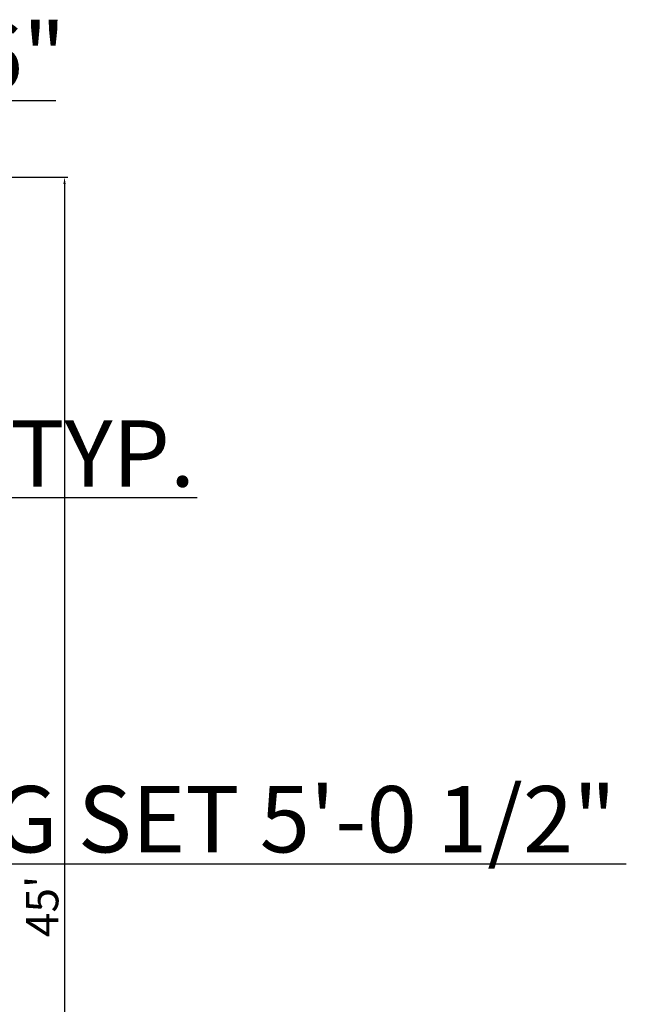
# Model space of a CAD drawing. Units: inches. Extents: x 1542 to 2523, y 1699 to 2449.
# Tile 7 of 7: x 2299 to 2523, y 1984 to 2349. Entities that reach past the tile are written whole.
import ezdxf

# ---------------------------------------------------------------- set-up
doc = ezdxf.new("R2010")
doc.units = ezdxf.units.IN
doc.layers.add('A-ANNO-DIMS', color=7, linetype='Continuous', lineweight=18)
doc.styles.get("Standard").update_dxf_attribs({"font": 'arial.ttf'})
doc.dimstyles.new('ISO-25', dxfattribs={"dimtxt": 24.5625, "dimasz": 2.5, "dimexe": 1.25, "dimexo": 0.625, "dimtad": 1, "dimlunit": 4, "dimtxsty": 'Standard', "dimcen": 2.5, "dimadec": 0, "dimazin": 0, "dimtfac": 10, "dimtmove": 0, "dimatfit": 3, "dimfxl": 1, "dimarcsym": 0})

# ---------------------------------------------------------------- blocks, each defined once
blk = doc.blocks.new('*D10')
at = {"layer": 'A-ANNO-DIMS', "color": 0, "lineweight": -2, "transparency": 16777216}
for p, q in [((2241.01, 2290.44), (2316.46, 2290.44)), ((2315.21, 2287.94), (2315.21, 1752.94)), ((2241.01, 1750.44), (2316.46, 1750.44))]:
    blk.add_line(p, q, dxfattribs=at)
at = {"layer": 'A-ANNO-DIMS', "color": 0, "transparency": 16777216}
for points in [[(2314.79, 2287.94), (2315.62, 2287.94), (2315.21, 2290.44)], [(2314.79, 1752.94), (2315.62, 1752.94), (2315.21, 1750.44)]]:
    blk.add_solid(points, dxfattribs=at)
at = {"layer": 'Defpoints', "color": 0, "transparency": 16777216}
for p in [(2240.38, 2290.44), (2240.38, 1750.44), (2315.21, 1750.44)]:
    blk.add_point(p, dxfattribs=at)
at = {"layer": 'A-ANNO-DIMS', "color": 0, "transparency": 16777216, "insert": (2308.48, 2020.44), "char_height": 12, "attachment_point": 5, "rotation": 90}
blk.add_mtext("45'", dxfattribs=at)
blk = doc.blocks.new('*D31')
at = {"layer": 'A-ANNO-DIMS', "color": 0, "lineweight": -2, "transparency": 16777216}
for p, q in [((2181.81, 2175.37), (2181.81, 2170.56)), ((2191.73, 2175.37), (2191.73, 2170.56)), ((2184.31, 2171.81), (2189.23, 2171.81)), ((2191.73, 2171.81), (2364.28, 2171.81))]:
    blk.add_line(p, q, dxfattribs=at)
at = {"layer": 'A-ANNO-DIMS', "color": 0, "transparency": 16777216}
for points in [[(2184.31, 2172.23), (2184.31, 2171.39), (2181.81, 2171.81)], [(2189.23, 2172.23), (2189.23, 2171.39), (2191.73, 2171.81)]]:
    blk.add_solid(points, dxfattribs=at)
at = {"layer": 'Defpoints', "color": 0, "transparency": 16777216}
for p in [(2181.81, 2175.99), (2191.73, 2175.99), (2191.73, 2171.81)]:
    blk.add_point(p, dxfattribs=at)
at = {"layer": 'A-ANNO-DIMS', "color": 0, "transparency": 16777216, "insert": (2279.26, 2184.97), "char_height": 24.5625, "attachment_point": 5}
blk.add_mtext('0\'-10" TYP.', dxfattribs=at)
blk = doc.blocks.new('*D42')
at = {"layer": 'A-ANNO-DIMS', "color": 0, "lineweight": -2, "transparency": 16777216}
for p, q in [((2131.75, 2027.78), (2131.75, 2037.46)), ((2134.25, 2036.21), (2189.62, 2036.21)), ((2192.12, 2027.78), (2192.12, 2037.46)), ((2192.12, 2036.21), (2523.07, 2036.21))]:
    blk.add_line(p, q, dxfattribs=at)
at = {"layer": 'A-ANNO-DIMS', "color": 0, "transparency": 16777216}
for points in [[(2134.25, 2036.63), (2134.25, 2035.8), (2131.75, 2036.21)], [(2189.62, 2036.63), (2189.62, 2035.8), (2192.12, 2036.21)]]:
    blk.add_solid(points, dxfattribs=at)
at = {"layer": 'Defpoints', "color": 0, "transparency": 16777216}
for p in [(2192.12, 2036.21), (2131.75, 2027.16), (2192.12, 2027.16)]:
    blk.add_point(p, dxfattribs=at)
at = {"layer": 'A-ANNO-DIMS', "color": 0, "transparency": 16777216, "insert": (2358.84, 2049.54), "char_height": 24.5625, "attachment_point": 5}
blk.add_mtext('DINING SET 5\'-0 1/2"', dxfattribs=at)
blk = doc.blocks.new('*D54')
at = {"layer": 'A-ANNO-DIMS', "color": 0, "lineweight": -2, "transparency": 16777216}
for p, q in [((2234.38, 2285.06), (2234.38, 2320.14)), ((2240.38, 2291.06), (2240.38, 2320.14)), ((2231.88, 2318.89), (2229.38, 2318.89)), ((2234.38, 2318.89), (2240.38, 2318.89)), ((2242.88, 2318.89), (2311.93, 2318.89))]:
    blk.add_line(p, q, dxfattribs=at)
at = {"layer": 'A-ANNO-DIMS', "color": 0, "transparency": 16777216}
for points in [[(2231.88, 2319.31), (2231.88, 2318.47), (2234.38, 2318.89)], [(2242.88, 2319.31), (2242.88, 2318.47), (2240.38, 2318.89)]]:
    blk.add_solid(points, dxfattribs=at)
at = {"layer": 'Defpoints', "color": 0, "transparency": 16777216}
for p in [(2240.38, 2318.89), (2240.38, 2290.44), (2234.38, 2284.44)]:
    blk.add_point(p, dxfattribs=at)
at = {"layer": 'A-ANNO-DIMS', "color": 0, "transparency": 16777216, "insert": (2278.65, 2332.05), "char_height": 24.562, "attachment_point": 5}
blk.add_mtext('0\'-6"', dxfattribs=at)

msp = doc.modelspace()

# ---------------------------------------------------------------- dimensions: what is measured, and where the dimension line sits
at = {"layer": 'A-ANNO-DIMS'}
dim = msp.add_linear_dim(base=(2240.383, 2318.889), p1=(2234.383, 2284.439), p2=(2240.383, 2290.439), dimstyle='ISO-25', override={"dimdec": 1, "dimlfac": 1, "dimrnd": 0, "dimzin": 1, "dimdsep": 46, "dimlunit": 4, "dimfrac": 2}, dxfattribs=at)
dim.commit()
dim.dimension.update_dxf_attribs({"geometry": '*D54', "text_midpoint": (2278.654, 2332.055)})
dim = msp.add_linear_dim(base=(2315.207, 1750.439), p1=(2240.383, 2290.439), p2=(2240.383, 1750.439), angle=90, dimstyle='ISO-25', override={"dimtxt": 12, "dimclrd": 0, "dimclre": 0, "dimclrt": 0}, dxfattribs=at)
dim.commit()
dim.dimension.update_dxf_attribs({"geometry": '*D10', "text_midpoint": (2308.48, 2020.439)})
for base, p1, p2, text, picture, middle in [((2191.731, 2171.809), (2181.813, 2175.993), (2191.731, 2175.993), '<> TYP.', '*D31', (2279.258, 2184.975)), ((2192.118, 2036.215), (2131.75, 2027.16), (2192.118, 2027.16), 'DINING SET <>', '*D42', (2358.845, 2049.54))]:
    dim = msp.add_linear_dim(base=base, p1=p1, p2=p2, text=text, dimstyle='ISO-25', override={"dimdec": 1, "dimlfac": 1, "dimrnd": 0, "dimzin": 1, "dimdsep": 46, "dimlunit": 4, "dimfrac": 2}, dxfattribs=at)
    dim.commit()
    dim.dimension.update_dxf_attribs({"geometry": picture, "text_midpoint": middle})

doc.saveas('drawing.dxf')
